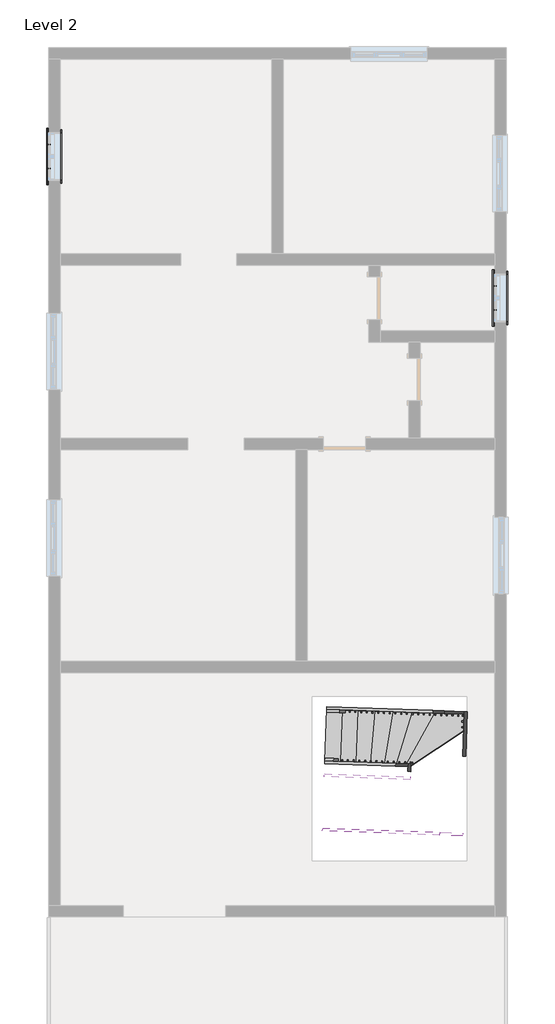
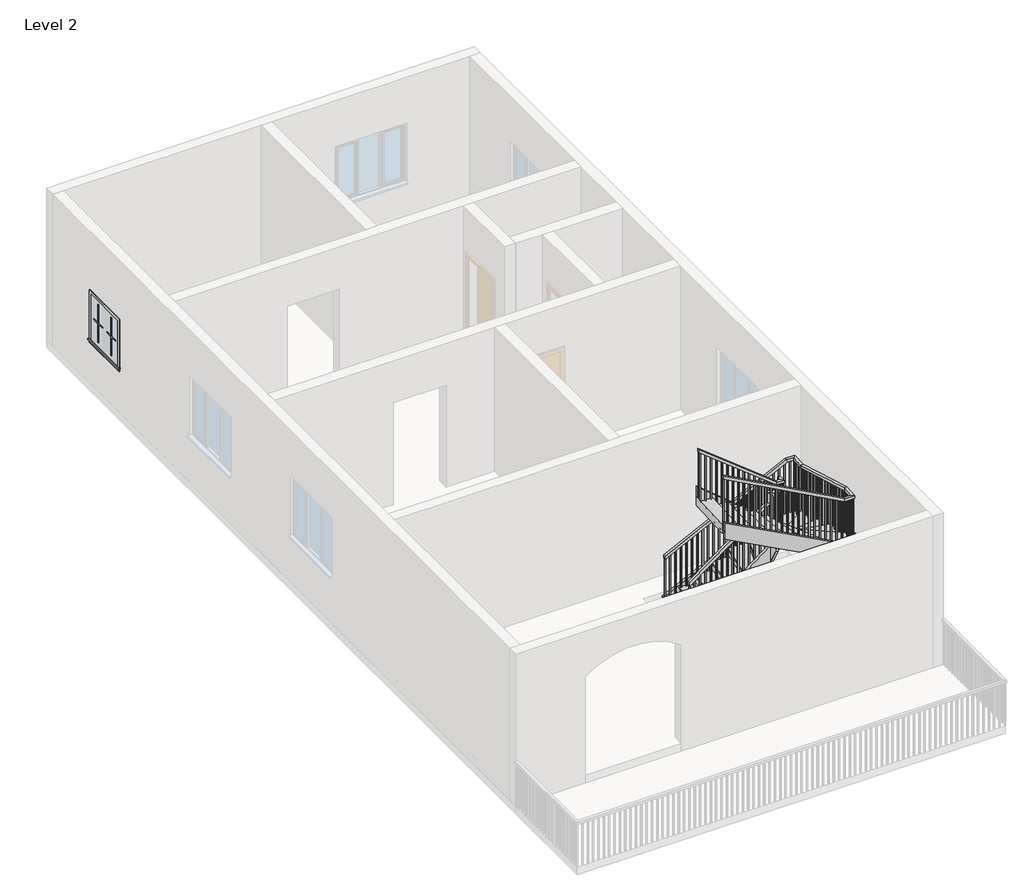
# One storey, part 3 of 3: 8 members, 8 proxies, 2 railings, 1 stair flight.
"""IFC4 building model written with IfcOpenShell, lengths in millimetres."""

from ifc_helpers import new_model, si_unit, frame, origin, place, context, project, spatial, polyline, outline, extrude, faceted_brep, transform, mapped, element, save
from components import muntin_pattern_2x2_muntin_pattern_2x2_b3fe6957, muntin_pattern_2x2_muntin_pattern_2x2_3e0ecaf2, trim_window_exterior_flat_with_sill_41619996, trim_window_interior_flat_picture_frame_51c85655, stair_flight_55d3e88d

model = new_model("IFC4")

# Units and contexts
model_context = context("Model", 3, world=origin())
ifc_project = project(units=[si_unit("LENGTHUNIT", "METRE", prefix="MILLI")], contexts=[model_context])

# Site, building, storey
site = spatial("IfcSite", under=ifc_project)
building = spatial("IfcBuilding", under=site)
storey = spatial("IfcBuildingStorey", under=building, Name="Level 2", Elevation=3048.0)

# Proxies
placement = place(None, origin())
muntin_pattern_2x2_muntin_pattern_2x2_shape = muntin_pattern_2x2_muntin_pattern_2x2_b3fe6957(model_context)
element("IfcBuildingElementProxy", 1, Name="Muntin Pattern_2x2 : Muntin Pattern_2x2", ObjectType="Muntin Pattern_2x2 : Muntin Pattern_2x2", at=placement, inside=storey, context=model_context, shape_type="MappedRepresentation", body=[
    mapped(muntin_pattern_2x2_muntin_pattern_2x2_shape, transform((-14939.9876504, 9248.016357, 4032.25), x_axis=(0.0, 1.0, 0.0), y_axis=(-1.0, 0.0, 0.0), z_axis=(0.0, 0.0, 1.0))),
])
element("IfcBuildingElementProxy", 2, Name="Muntin Pattern_2x2 : Muntin Pattern_2x2", ObjectType="Muntin Pattern_2x2 : Muntin Pattern_2x2", at=placement, inside=storey, context=model_context, shape_type="MappedRepresentation", body=[
    mapped(muntin_pattern_2x2_muntin_pattern_2x2_shape, transform((-7015.1876504, 6733.416357, 4032.25), x_axis=(0.0, 1.0, 0.0), y_axis=(-1.0, 0.0, 0.0), z_axis=(0.0, 0.0, 1.0))),
])
muntin_pattern_2x2_muntin_pattern_2x2_2_shape = muntin_pattern_2x2_muntin_pattern_2x2_3e0ecaf2(model_context)
element("IfcBuildingElementProxy", 3, Name="Muntin Pattern_2x2 : Muntin Pattern_2x2", ObjectType="Muntin Pattern_2x2 : Muntin Pattern_2x2", at=placement, inside=storey, context=model_context, shape_type="MappedRepresentation", body=[
    mapped(muntin_pattern_2x2_muntin_pattern_2x2_2_shape, transform((-14939.9876504, 9676.641357, 4032.25), x_axis=(0.0, -1.0, 0.0), y_axis=(1.0, 0.0, 0.0), z_axis=(0.0, 0.0, 1.0))),
])
element("IfcBuildingElementProxy", 4, Name="Muntin Pattern_2x2 : Muntin Pattern_2x2", ObjectType="Muntin Pattern_2x2 : Muntin Pattern_2x2", at=placement, inside=storey, context=model_context, shape_type="MappedRepresentation", body=[
    mapped(muntin_pattern_2x2_muntin_pattern_2x2_2_shape, transform((-7015.1876504, 7162.041357, 4032.25), x_axis=(0.0, -1.0, 0.0), y_axis=(1.0, 0.0, 0.0), z_axis=(0.0, 0.0, 1.0))),
])
trim_window_exterior_flat_with_sill_shape = trim_window_exterior_flat_with_sill_41619996(model_context)
element("IfcBuildingElementProxy", 5, Name="Trim-Window-Exterior-Flat : with Sill", ObjectType="Trim-Window-Exterior-Flat : with Sill", at=placement, inside=storey, context=model_context, shape_type="MappedRepresentation", body=[
    mapped(trim_window_exterior_flat_with_sill_shape, transform((-14949.5126504, 9462.328857, 4876.8), x_axis=(0.0, -1.0, 0.0), y_axis=(0.0, 0.0, 1.0), z_axis=(-1.0, 0.0, 0.0))),
])
element("IfcBuildingElementProxy", 6, Name="Trim-Window-Exterior-Flat : with Sill", ObjectType="Trim-Window-Exterior-Flat : with Sill", at=placement, inside=storey, context=model_context, shape_type="MappedRepresentation", body=[
    mapped(trim_window_exterior_flat_with_sill_shape, transform((-7024.7126504, 6947.728857, 4876.8), x_axis=(0.0, -1.0, 0.0), y_axis=(0.0, 0.0, 1.0), z_axis=(-1.0, 0.0, 0.0))),
])
trim_window_interior_flat_picture_frame_shape = trim_window_interior_flat_picture_frame_51c85655(model_context)
element("IfcBuildingElementProxy", 7, Name="Trim-Window-Interior-Flat : Picture Frame", ObjectType="Trim-Window-Interior-Flat : Picture Frame", at=placement, inside=storey, context=model_context, shape_type="MappedRepresentation", body=[
    mapped(trim_window_interior_flat_picture_frame_shape, transform((-14746.3126504, 9462.328857, 4876.8), x_axis=(0.0, 1.0, 0.0), y_axis=(0.0, 0.0, 1.0), z_axis=(1.0, 0.0, 0.0))),
])
element("IfcBuildingElementProxy", 8, Name="Trim-Window-Interior-Flat : Picture Frame", ObjectType="Trim-Window-Interior-Flat : Picture Frame", at=placement, inside=storey, context=model_context, shape_type="MappedRepresentation", body=[
    mapped(trim_window_interior_flat_picture_frame_shape, transform((-6821.5126504, 6947.728857, 4876.8), x_axis=(0.0, 1.0, 0.0), y_axis=(0.0, 0.0, 1.0), z_axis=(1.0, 0.0, 0.0))),
])

# Members
element("IfcMember", 9, ObjectType="Stringer - 2\" Width", at=placement, inside=storey, context=model_context, shape_type="SweptSolid", body=[
    extrude(outline(polyline([(157.0794453, -304.8), (51.8818925, -100.6726296), (247.2290139, 0.0), (2348.3102094, 0.0), (2505.3896547, -304.8), (157.0794453, -304.8)])), frame((-10006.394185, -363.3128759, 2934.7449378), z_axis=(0.03595828761805288, 0.9993532916599501, 0.0), x_axis=(0.8883269481492082, -0.03196338688929392, 0.4580977789626134)), (0.0, 0.0, 1.0), 50.8),
])
element("IfcMember", 10, ObjectType="Stringer - 2\" Width", at=placement, inside=storey, context=model_context, shape_type="SweptSolid", body=[
    extrude(outline(polyline([(-7920.3269434, -438.3728236), (-7918.5002624, -387.6056764), (-7564.0151591, -400.3606025), (-7565.8418401, -451.1277497), (-7920.3269434, -438.3728236)])), frame((0.0, 0.0, 4010.500629), z_axis=(0.0, 0.0, 1.0), x_axis=(1.0, 0.0, 0.0)), (0.0, 0.0, 1.0), 342.8950162),
])
element("IfcMember", 11, ObjectType="Stringer - 2\" Width", at=placement, inside=storey, context=model_context, shape_type="SweptSolid", body=[
    extrude(outline(polyline([(-141.4966894, -274.7041443), (-53.351137, 0.0), (2175.2349578, 0.0), (2210.4467651, -11.2985708), (2109.3071449, -326.4985112), (19.9195916, -326.4985112), (-141.4966894, -274.7041443)])), frame((-7515.0746928, -452.9544307, 4353.3956453), z_axis=(-0.9993532916599501, 0.035958287618053086, 0.0), x_axis=(-0.03423883934699899, -0.9515663584286186, 0.3055309597848772)), (0.0, 0.0, 1.0), 50.8),
])
element("IfcMember", 12, ObjectType="Stringer - 2\" Width", at=placement, inside=storey, context=model_context, shape_type="SweptSolid", body=[
    extrude(outline(polyline([(-7590.8819548, -2559.7910402), (-7592.7086358, -2610.5581874), (-7997.9608864, -2595.9765803), (-7996.1342054, -2545.2094331), (-7590.8819548, -2559.7910402)])), frame((0.0, 0.0, 4697.8904473), z_axis=(0.0, 0.0, 1.0), x_axis=(1.0, 0.0, 0.0)), (0.0, 0.0, 1.0), 320.1068224),
])
element("IfcMember", 13, ObjectType="Stringer - 2\" Width", at=placement, inside=storey, context=model_context, shape_type="SweptSolid", body=[
    extrude(outline(polyline([(-146.6402244, -284.5435333), (0.0, 0.0), (2348.3102094, 0.0), (2201.669985, -284.5435333), (-146.6402244, -284.5435333)])), frame((-7997.9608864, -2595.9765803, 5017.9972697), z_axis=(0.03595828761805283, 0.9993532916599502, 0.0), x_axis=(-0.8883269481492087, 0.03196338688929389, 0.45809777896261245)), (0.0, 0.0, 1.0), 50.8),
])
element("IfcMember", 14, ObjectType="Stringer - 2\" Width", at=placement, inside=storey, context=model_context, shape_type="SweptSolid", body=[
    extrude(outline(polyline([(248.5240347, -304.8), (137.1927864, -168.2588219), (343.5522597, 0.0), (1905.6564494, 0.0), (2154.1804842, -304.8), (248.5240347, -304.8)])), frame((-10041.1011242, -1327.888673, 2830.8988904), z_axis=(0.03595828761805293, 0.9993532916599501, 0.0), x_axis=(0.7745239433168307, -0.02786857756239004, 0.6319303787709498)), (0.0, 0.0, 1.0), 50.8),
])
element("IfcMember", 15, ObjectType="Stringer - 2\" Width", at=placement, inside=storey, context=model_context, shape_type="SweptSolid", body=[
    extrude(outline(polyline([(-470.0446027, -275.2513009), (0.0, 0.0), (408.9230004, 1e-07), (420.0212921, -18.9524702), (-68.1184117, -304.7999999), (-452.7413132, -304.8), (-470.0446027, -275.2513009)])), frame((-8512.5307482, -1332.0561414, 4621.2682978), z_axis=(-0.9993532916599503, 0.03595828761805068, 0.0), x_axis=(-0.018170454813323342, -0.5049935642524197, 0.8629318250218347)), (0.0, 0.0, 1.0), 50.8),
])
element("IfcMember", 16, ObjectType="Stringer - 2\" Width", at=placement, inside=storey, context=model_context, shape_type="SweptSolid", body=[
    extrude(outline(polyline([(-248.5240348, -304.8), (0.0, 0.0), (1971.2027087, 0.0), (1722.6786739, -304.8), (-248.5240348, -304.8)])), frame((-8522.5774937, -1611.2754511, 4974.1409689), z_axis=(0.0359582876180528, 0.9993532916599502, 0.0), x_axis=(-0.7745239433168305, 0.027868577562389935, 0.63193037877095)), (0.0, 0.0, 1.0), 50.8),
])

# Railings
element("IfcRailing", 17, ObjectType="Handrail - Rectangular", at=placement, inside=storey, context=model_context, shape_type="SolidModel", body=[
    faceted_brep([(-10037.4477622, -1226.3543786, 4131.7333333), (-10037.4477622, -1226.3543786, 4067.4000346), (-10039.2744432, -1277.1215258, 4067.4000346), (-10039.2744432, -1277.1215258, 4131.7333333), (-8586.854788, -1278.5489726, 5259.6191036), (-8536.0876408, -1280.3756536, 5234.7590024), (-8537.9143218, -1331.1428009, 5234.7590024), (-8588.681469, -1329.3161198, 5259.6191036), (-8586.854788, -1278.5489726, 5462.6281882), (-8536.0876408, -1280.3756536, 5411.8281882), (-8537.9143218, -1331.1428009, 5411.8281882), (-8588.681469, -1329.3161198, 5462.6281882), (-8459.9369199, -1283.1156752, 5462.6281882), (-8459.9369199, -1283.1156752, 5411.8281882), (-8512.5307482, -1332.0561414, 5411.8281882), (-8512.5307482, -1332.0561414, 5462.6281882), (-8464.5036225, -1410.0335432, 5462.6281882), (-8465.5507758, -1439.136044, 5411.8281882), (-8516.317923, -1437.309363, 5411.8281882), (-8515.2707697, -1408.2068622, 5462.6281882), (-8469.070325, -1536.9514112, 5679.5051451), (-8470.897006, -1587.7185585, 5665.7256424), (-8521.6641532, -1585.8918774, 5665.7256424), (-8519.8374722, -1535.1247302, 5679.5051451), (-8469.070325, -1536.9514112, 5882.5142297), (-8470.897006, -1587.7185585, 5831.7142297), (-8521.6641532, -1585.8918774, 5831.7142297), (-8519.8374722, -1535.1247302, 5882.5142297), (-8473.6370275, -1663.8692793, 5882.5142297), (-8473.6370275, -1663.8692793, 5831.7142297), (-8522.5774937, -1611.2754511, 5831.7142297), (-8522.5774937, -1611.2754511, 5882.5142297), (-8600.5548956, -1659.3025768, 5882.5142297), (-8617.9603, -1658.6763032, 5831.7142297), (-8616.133619, -1607.909156, 5831.7142297), (-8598.7282145, -1608.5354295, 5882.5142297), (-10051.1478698, -1607.1079827, 7010.4), (-10049.3211887, -1556.3408355, 7010.4), (-10049.3211887, -1556.3408355, 6946.0667013), (-10051.1478698, -1607.1079827, 6946.0667013)], [[[0, 1, 2, 3]], [[1, 0, 4, 5]], [[2, 1, 5, 6]], [[3, 2, 6, 7]], [[0, 3, 7, 4]], [[5, 4, 8, 9]], [[6, 5, 9, 10]], [[7, 6, 10, 11]], [[4, 7, 11, 8]], [[9, 8, 12, 13]], [[10, 9, 13, 14]], [[11, 10, 14, 15]], [[8, 11, 15, 12]], [[13, 12, 16, 17]], [[14, 13, 17, 18]], [[15, 14, 18, 19]], [[12, 15, 19, 16]], [[17, 16, 20, 21]], [[18, 17, 21, 22]], [[19, 18, 22, 23]], [[16, 19, 23, 20]], [[21, 20, 24, 25]], [[22, 21, 25, 26]], [[23, 22, 26, 27]], [[20, 23, 27, 24]], [[25, 24, 28, 29]], [[26, 25, 29, 30]], [[27, 26, 30, 31]], [[24, 27, 31, 28]], [[29, 28, 32, 33]], [[30, 29, 33, 34]], [[31, 30, 34, 35]], [[28, 31, 35, 32]], [[36, 37, 38, 39]], [[33, 32, 36, 39]], [[34, 33, 39, 38]], [[35, 34, 38, 37]], [[32, 35, 37, 36]]]),
    extrude(outline(polyline([(236.0012245, -19.05), (221.1987754, 0.0), (1225.3637939, 0.0), (1225.3637939, -19.05), (236.0012245, -19.05)])), frame((-10030.9830199, -1591.9482723, 7152.0304606), z_axis=(0.0359582876180528, 0.9993532916599503, 0.0), x_axis=(0.0, 0.0, -1.0)), (0.0, 0.0, 1.0), 19.05),
    extrude(outline(polyline([(236.0012246, -19.05), (221.1987755, 0.0), (1146.417399, 0.0), (1146.417399, -19.05), (236.0012246, -19.05)])), frame((-9929.4487255, -1595.6016343, 7073.0840657), z_axis=(0.0359582876180528, 0.9993532916599503, 0.0), x_axis=(0.0, 0.0, -1.0)), (0.0, 0.0, 1.0), 19.05),
    extrude(outline(polyline([(236.0012245, -19.05), (221.1987755, 0.0), (1067.471004, 0.0), (1067.471004, -19.05), (236.0012245, -19.05)])), frame((-9827.914431, -1599.2549963, 6994.1376707), z_axis=(0.0359582876180528, 0.9993532916599503, 0.0), x_axis=(0.0, 0.0, -1.0)), (0.0, 0.0, 1.0), 19.05),
    extrude(outline(polyline([(236.0012245, -19.05), (221.1987754, 0.0), (1157.8579424, 0.0), (1157.8579424, -19.05), (236.0012245, -19.05)])), frame((-9726.3801366, -1602.9083583, 6915.1912757), z_axis=(0.0359582876180528, 0.9993532916599503, 0.0), x_axis=(0.0, 0.0, -1.0)), (0.0, 0.0, 1.0), 19.05),
    extrude(outline(polyline([(236.0012246, -19.05), (221.1987755, 0.0), (1078.9115475, 0.0), (1078.9115475, -19.05), (236.0012246, -19.05)])), frame((-9624.8458422, -1606.5617203, 6836.2448808), z_axis=(0.0359582876180528, 0.9993532916599503, 0.0), x_axis=(0.0, 0.0, -1.0)), (0.0, 0.0, 1.0), 19.05),
    extrude(outline(polyline([(236.0012245, -19.05), (221.1987755, 0.0), (999.9651525, 0.0), (999.9651525, -19.05), (236.0012245, -19.05)])), frame((-9523.3115477, -1610.2150824, 6757.2984858), z_axis=(0.0359582876180528, 0.9993532916599503, 0.0), x_axis=(0.0, 0.0, -1.0)), (0.0, 0.0, 1.0), 19.05),
    extrude(outline(polyline([(236.0012245, -19.05), (221.1987754, 0.0), (1090.3520908, 0.0), (1090.3520908, -19.05), (236.0012245, -19.05)])), frame((-9421.7772533, -1613.8684444, 6678.3520908), z_axis=(0.0359582876180528, 0.9993532916599503, 0.0), x_axis=(0.0, 0.0, -1.0)), (0.0, 0.0, 1.0), 19.05),
    extrude(outline(polyline([(236.0012246, -19.05), (221.1987755, 0.0), (1011.4056959, 0.0), (1011.4056959, -19.05), (236.0012246, -19.05)])), frame((-9320.2429589, -1617.5218064, 6599.4056959), z_axis=(0.0359582876180528, 0.9993532916599503, 0.0), x_axis=(0.0, 0.0, -1.0)), (0.0, 0.0, 1.0), 19.05),
    extrude(outline(polyline([(236.0012245, -19.05), (221.1987755, 0.0), (1101.7926342, 0.0), (1101.7926342, -19.05), (236.0012245, -19.05)])), frame((-9218.7086644, -1621.1751684, 6520.4593009), z_axis=(0.0359582876180528, 0.9993532916599503, 0.0), x_axis=(0.0, 0.0, -1.0)), (0.0, 0.0, 1.0), 19.05),
    extrude(outline(polyline([(236.0012245, -19.05), (221.1987755, 0.0), (1022.8462392, 0.0), (1022.8462392, -19.05), (236.0012245, -19.05)])), frame((-9117.17437, -1624.8285304, 6441.5129059), z_axis=(0.0359582876180528, 0.9993532916599503, 0.0), x_axis=(0.0, 0.0, -1.0)), (0.0, 0.0, 1.0), 19.05),
    extrude(outline(polyline([(236.0012245, -19.05), (221.1987754, 0.0), (943.8998442, 0.0), (943.8998442, -19.05), (236.0012245, -19.05)])), frame((-9015.6400756, -1628.4818925, 6362.5665109), z_axis=(0.0359582876180528, 0.9993532916599503, 0.0), x_axis=(0.0, 0.0, -1.0)), (0.0, 0.0, 1.0), 19.05),
    extrude(outline(polyline([(236.0012246, -19.05), (221.1987755, 0.0), (1034.2867827, 0.0), (1034.2867827, -19.05), (236.0012246, -19.05)])), frame((-8914.1057811, -1632.1352545, 6283.620116), z_axis=(0.0359582876180528, 0.9993532916599503, 0.0), x_axis=(0.0, 0.0, -1.0)), (0.0, 0.0, 1.0), 19.05),
    extrude(outline(polyline([(236.0012245, -19.05), (221.1987755, 0.0), (955.3403877, 0.0), (955.3403877, -19.05), (236.0012245, -19.05)])), frame((-8812.5714867, -1635.7886165, 6204.673721), z_axis=(0.0359582876180528, 0.9993532916599503, 0.0), x_axis=(0.0, 0.0, -1.0)), (0.0, 0.0, 1.0), 19.05),
    extrude(outline(polyline([(236.0012245, -19.05), (221.1987754, 0.0), (1045.727326, 0.0), (1045.727326, -19.05), (236.0012245, -19.05)])), frame((-8711.0371923, -1639.4419785, 6125.727326), z_axis=(0.0359582876180528, 0.9993532916599503, 0.0), x_axis=(0.0, 0.0, -1.0)), (0.0, 0.0, 1.0), 19.05),
    extrude(outline(polyline([(236.0012246, -19.05), (221.1987755, 0.0), (966.7809311, 0.0), (966.7809311, -19.05), (236.0012246, -19.05)])), frame((-8609.5028978, -1643.0953406, 6046.7809311), z_axis=(0.0359582876180528, 0.9993532916599503, 0.0), x_axis=(0.0, 0.0, -1.0)), (0.0, 0.0, 1.0), 19.05),
    extrude(outline(polyline([(-8506.3702575, -1602.3274488), (-8487.3325773, -1603.0124541), (-8488.0175827, -1622.0501344), (-8507.0552629, -1621.365129), (-8506.3702575, -1602.3274488)])), frame((0.0, 0.0, 4741.3333333), z_axis=(0.0, 0.0, 1.0), x_axis=(1.0, 0.0, 0.0)), (0.0, 0.0, 1.0), 1090.3808964),
    extrude(outline(polyline([(244.8657718, -19.05), (212.3342282, 0.0), (1192.1994682, 0.0), (1192.1994682, -19.05), (244.8657718, -19.05)])), frame((-8484.3642207, -1520.5158399, 5764.1994682), z_axis=(-0.9993532916599502, 0.035958287618050686, 0.0), x_axis=(0.0, 0.0, -1.0)), (0.0, 0.0, 1.0), 19.05),
    extrude(outline(polyline([(244.8657717, -19.05), (212.3342282, 0.0), (1188.0312359, 0.0), (1188.0312359, -19.05), (244.8657717, -19.05)])), frame((-8480.7108586, -1418.9815455, 5590.6979026), z_axis=(-0.9993532916599502, 0.035958287618050686, 0.0), x_axis=(0.0, 0.0, -1.0)), (0.0, 0.0, 1.0), 19.05),
    extrude(outline(polyline([(-8525.208029, -1315.7147199), (-8524.5230236, -1296.6770397), (-8505.4853434, -1297.3620451), (-8506.1703488, -1316.3997253), (-8525.208029, -1315.7147199)])), frame((0.0, 0.0, 4233.3333333), z_axis=(0.0, 0.0, 1.0), x_axis=(1.0, 0.0, 0.0)), (0.0, 0.0, 1.0), 1178.4948549),
    extrude(outline(polyline([(221.1987754, -19.05), (236.0012245, 0.0), (1337.2495642, 0.0), (1337.2495642, -19.05), (221.1987754, -19.05)])), frame((-8626.7423234, -1312.0613579, 5401.2495642), z_axis=(0.035958287618052934, 0.9993532916599503, 0.0), x_axis=(0.0, 0.0, -1.0)), (0.0, 0.0, 1.0), 19.05),
    extrude(outline(polyline([(221.1987755, -19.0500001), (236.0012246, 0.0), (1258.3031693, 0.0), (1258.3031693, -19.0500001), (221.1987755, -19.0500001)])), frame((-8728.2766179, -1308.4079959, 5322.3031693), z_axis=(0.035958287618052934, 0.9993532916599503, 0.0), x_axis=(0.0, 0.0, -1.0)), (0.0, 0.0, 1.0), 19.05),
    extrude(outline(polyline([(221.1987755, -19.05), (236.0012245, 0.0), (1348.6901076, 0.0), (1348.6901076, -19.05), (221.1987755, -19.05)])), frame((-8829.8109123, -1304.7546339, 5243.3567743), z_axis=(0.035958287618052934, 0.9993532916599503, 0.0), x_axis=(0.0, 0.0, -1.0)), (0.0, 0.0, 1.0), 19.05),
    extrude(outline(polyline([(221.1987754, -19.05), (236.0012245, 0.0), (1269.7437126, 0.0), (1269.7437126, -19.05), (221.1987754, -19.05)])), frame((-8931.3452067, -1301.1012718, 5164.4103793), z_axis=(0.035958287618052934, 0.9993532916599503, 0.0), x_axis=(0.0, 0.0, -1.0)), (0.0, 0.0, 1.0), 19.05),
    extrude(outline(polyline([(221.1987755, -19.05), (236.0012246, 0.0), (1360.1306511, 0.0), (1360.1306511, -19.05), (221.1987755, -19.05)])), frame((-9032.8795011, -1297.4479098, 5085.4639844), z_axis=(0.035958287618052934, 0.9993532916599503, 0.0), x_axis=(0.0, 0.0, -1.0)), (0.0, 0.0, 1.0), 19.05),
    extrude(outline(polyline([(221.1987755, -19.05), (236.0012245, 0.0), (1281.1842561, 0.0), (1281.1842561, -19.05), (221.1987755, -19.05)])), frame((-9134.4137956, -1293.7945478, 5006.5175894), z_axis=(0.035958287618052934, 0.9993532916599503, 0.0), x_axis=(0.0, 0.0, -1.0)), (0.0, 0.0, 1.0), 19.05),
    extrude(outline(polyline([(221.1987755, -19.05), (236.0012245, 0.0), (1371.5711944, 0.0), (1371.5711944, -19.05), (221.1987755, -19.05)])), frame((-9235.94809, -1290.1411858, 4927.5711944), z_axis=(0.035958287618052934, 0.9993532916599503, 0.0), x_axis=(0.0, 0.0, -1.0)), (0.0, 0.0, 1.0), 19.05),
    extrude(outline(polyline([(221.1987754, -19.05), (236.0012245, 0.0), (1292.6247994, 0.0), (1292.6247994, -19.05), (221.1987754, -19.05)])), frame((-9337.4823844, -1286.4878237, 4848.6247994), z_axis=(0.035958287618052934, 0.9993532916599503, 0.0), x_axis=(0.0, 0.0, -1.0)), (0.0, 0.0, 1.0), 19.05),
    extrude(outline(polyline([(221.1987755, -19.05), (236.0012246, 0.0), (1213.6784045, 0.0), (1213.6784045, -19.05), (221.1987755, -19.05)])), frame((-9439.0166789, -1282.8344617, 4769.6784045), z_axis=(0.035958287618052934, 0.9993532916599503, 0.0), x_axis=(0.0, 0.0, -1.0)), (0.0, 0.0, 1.0), 19.05),
    extrude(outline(polyline([(221.1987755, -19.05), (236.0012245, 0.0), (1304.0653428, 0.0), (1304.0653428, -19.05), (221.1987755, -19.05)])), frame((-9540.5509733, -1279.1810997, 4690.7320095), z_axis=(0.035958287618052934, 0.9993532916599503, 0.0), x_axis=(0.0, 0.0, -1.0)), (0.0, 0.0, 1.0), 19.05),
    extrude(outline(polyline([(221.1987754, -19.05), (236.0012245, 0.0), (1225.1189478, 0.0), (1225.1189478, -19.05), (221.1987754, -19.05)])), frame((-9642.0852677, -1275.5277377, 4611.7856145), z_axis=(0.035958287618052934, 0.9993532916599503, 0.0), x_axis=(0.0, 0.0, -1.0)), (0.0, 0.0, 1.0), 19.05),
    extrude(outline(polyline([(221.1987755, -19.05), (236.0012246, 0.0), (1146.1725529, 0.0), (1146.1725529, -19.05), (221.1987755, -19.05)])), frame((-9743.6195622, -1271.8743757, 4532.8392196), z_axis=(0.035958287618052934, 0.9993532916599503, 0.0), x_axis=(0.0, 0.0, -1.0)), (0.0, 0.0, 1.0), 19.05),
    extrude(outline(polyline([(221.1987755, -19.05), (236.0012245, 0.0), (1236.5594913, 0.0), (1236.5594913, -19.05), (221.1987755, -19.05)])), frame((-9845.1538566, -1268.2210136, 4453.8928246), z_axis=(0.035958287618052934, 0.9993532916599503, 0.0), x_axis=(0.0, 0.0, -1.0)), (0.0, 0.0, 1.0), 19.05),
    extrude(outline(polyline([(221.1987755, -19.05), (236.0012245, 0.0), (1157.6130963, 0.0), (1157.6130963, -19.05), (221.1987755, -19.05)])), frame((-9946.688151, -1264.5676516, 4374.9464296), z_axis=(0.035958287618052934, 0.9993532916599503, 0.0), x_axis=(0.0, 0.0, -1.0)), (0.0, 0.0, 1.0), 19.05),
    extrude(outline(polyline([(-8507.283598, -1627.7110224), (-8488.2459178, -1628.3960278), (-8488.9309232, -1647.433708), (-8507.9686034, -1646.7487026), (-8507.283598, -1627.7110224)])), frame((0.0, 0.0, 4910.6666667), z_axis=(0.0, 0.0, 1.0), x_axis=(1.0, 0.0, 0.0)), (0.0, 0.0, 1.0), 921.0475631),
    extrude(outline(polyline([(-8496.0951768, -1316.7622457), (-8495.4101715, -1297.7245655), (-8476.3724912, -1298.4095708), (-8477.0574966, -1317.4472511), (-8496.0951768, -1316.7622457)])), frame((0.0, 0.0, 4233.3333333), z_axis=(0.0, 0.0, 1.0), x_axis=(1.0, 0.0, 0.0)), (0.0, 0.0, 1.0), 1178.4948549),
    extrude(outline(polyline([(236.0012245, -19.05), (221.1987755, 0.0), (1240.5988101, 0.0), (1240.5988101, -19.05), (236.0012245, -19.05)])), frame((-10050.5770319, -1591.2432492, 7167.2654768), z_axis=(0.0359582876180528, 0.9993532916599503, 0.0), x_axis=(0.0, 0.0, -1.0)), (0.0, 0.0, 1.0), 19.05),
    extrude(outline(polyline([(221.1987755, -19.05), (236.0012246, 0.0), (1086.0679259, 0.0), (1086.0679259, -19.05), (221.1987755, -19.05)])), frame((-10038.7036054, -1261.2567923, 4303.4012592), z_axis=(0.035958287618052934, 0.9993532916599503, 0.0), x_axis=(0.0, 0.0, -1.0)), (0.0, 0.0, 1.0), 19.05),
])
element("IfcRailing", 18, ObjectType="Handrail - Rectangular", at=placement, inside=storey, context=model_context, shape_type="SolidModel", body=[
    faceted_brep([(-10006.394185, -363.3128759, 4131.7333333), (-10006.394185, -363.3128759, 4074.2742652), (-10008.220866, -414.0800231, 4074.2742652), (-10008.220866, -414.0800231, 4131.7333333), (-7750.1292126, -444.496803, 5325.0239201), (-7737.5382959, -444.9498438, 5274.2239201), (-7739.364977, -495.716991, 5274.2239201), (-7751.9558936, -495.2639503, 5325.0239201), (-7565.8418401, -451.1277497, 5325.0239201), (-7565.8418401, -451.1277497, 5274.2239201), (-7618.4356683, -500.0682159, 5274.2239201), (-7618.4356683, -500.0682159, 5325.0239201), (-7576.1730834, -738.2538248, 5325.0239201), (-7576.4589725, -746.1992592, 5274.2239201), (-7627.2261197, -744.3725782, 5274.2239201), (-7626.9402306, -736.4271438, 5325.0239201), (-7631.3178587, -2270.838284, 5817.1094132), (-7631.6037478, -2278.7837184, 5766.3094132), (-7682.370895, -2276.9570374, 5766.3094132), (-7682.0850059, -2269.011603, 5817.1094132), (-7641.649102, -2557.9643591, 5817.1094132), (-7641.649102, -2557.9643591, 5766.3094132), (-7690.5895682, -2505.3705309, 5766.3094132), (-7690.5895682, -2505.3705309, 5817.1094132), (-7825.9364745, -2551.3334125, 5817.1094132), (-7838.5273911, -2550.8803717, 5766.3094132), (-7836.7007101, -2500.1132245, 5766.3094132), (-7824.1097935, -2500.5662653, 5817.1094132), (-10082.2014469, -2470.1494854, 7010.4), (-10080.3747659, -2419.3823382, 7010.4), (-10080.3747659, -2419.3823382, 6952.9409318), (-10082.2014469, -2470.1494854, 6952.9409318)], [[[0, 1, 2, 3]], [[1, 0, 4, 5]], [[2, 1, 5, 6]], [[3, 2, 6, 7]], [[0, 3, 7, 4]], [[5, 4, 8, 9]], [[6, 5, 9, 10]], [[7, 6, 10, 11]], [[4, 7, 11, 8]], [[9, 8, 12, 13]], [[10, 9, 13, 14]], [[11, 10, 14, 15]], [[8, 11, 15, 12]], [[13, 12, 16, 17]], [[14, 13, 17, 18]], [[15, 14, 18, 19]], [[12, 15, 19, 16]], [[17, 16, 20, 21]], [[18, 17, 21, 22]], [[19, 18, 22, 23]], [[16, 19, 23, 20]], [[21, 20, 24, 25]], [[22, 21, 25, 26]], [[23, 22, 26, 27]], [[20, 23, 27, 24]], [[28, 29, 30, 31]], [[25, 24, 28, 31]], [[26, 25, 31, 30]], [[27, 26, 30, 29]], [[24, 27, 29, 28]]]),
    extrude(outline(polyline([(223.5656878, 19.05), (1212.6274313, 19.05), (1212.6274313, 0.0), (233.6343122, 0.0), (223.5656878, 19.05)])), frame((-9992.2317697, -2457.5014613, 7139.294098), z_axis=(0.035958287618052934, 0.9993532916599503, 0.0), x_axis=(0.0, 0.0, -1.0)), (0.0, 0.0, 1.0), 19.05),
    extrude(outline(polyline([(223.5656878, 19.05), (1158.9281011, 19.05), (1158.9281011, 0.0), (233.6343122, 0.0), (223.5656878, 19.05)])), frame((-9890.6974752, -2461.1548233, 7085.5947678), z_axis=(0.035958287618052934, 0.9993532916599503, 0.0), x_axis=(0.0, 0.0, -1.0)), (0.0, 0.0, 1.0), 19.05),
    extrude(outline(polyline([(223.5656878, 19.05), (1274.5621043, 19.05), (1274.5621043, 0.0), (233.6343122, 0.0), (223.5656878, 19.05)])), frame((-9789.1631808, -2464.8081854, 7031.8954376), z_axis=(0.035958287618052934, 0.9993532916599503, 0.0), x_axis=(0.0, 0.0, -1.0)), (0.0, 0.0, 1.0), 19.05),
    extrude(outline(polyline([(223.5656878, 19.05), (1220.8627741, 19.05), (1220.8627741, 0.0), (233.6343122, 0.0), (223.5656878, 19.05)])), frame((-9687.6288864, -2468.4615474, 6978.1961074), z_axis=(0.035958287618052934, 0.9993532916599503, 0.0), x_axis=(0.0, 0.0, -1.0)), (0.0, 0.0, 1.0), 19.05),
    extrude(outline(polyline([(223.5656878, 19.05), (1167.1634439, 19.05), (1167.1634439, 0.0), (233.6343122, 0.0), (223.5656878, 19.05)])), frame((-9586.0945919, -2472.1149094, 6924.4967772), z_axis=(0.035958287618052934, 0.9993532916599503, 0.0), x_axis=(0.0, 0.0, -1.0)), (0.0, 0.0, 1.0), 19.05),
    extrude(outline(polyline([(223.5656878, 19.05), (1282.797447, 19.05), (1282.797447, 0.0), (233.6343122, 0.0), (223.5656878, 19.05)])), frame((-9484.5602975, -2475.7682714, 6870.797447), z_axis=(0.035958287618052934, 0.9993532916599503, 0.0), x_axis=(0.0, 0.0, -1.0)), (0.0, 0.0, 1.0), 19.05),
    extrude(outline(polyline([(223.5656878, 19.05), (1229.0981168, 19.05), (1229.0981168, 0.0), (233.6343122, 0.0), (223.5656878, 19.05)])), frame((-9383.0260031, -2479.4216334, 6817.0981168), z_axis=(0.035958287618052934, 0.9993532916599503, 0.0), x_axis=(0.0, 0.0, -1.0)), (0.0, 0.0, 1.0), 19.05),
    extrude(outline(polyline([(223.5656878, 19.05), (1175.3987866, 19.05), (1175.3987866, 0.0), (233.6343122, 0.0), (223.5656878, 19.05)])), frame((-9281.4917086, -2483.0749955, 6763.3987866), z_axis=(0.035958287618052934, 0.9993532916599503, 0.0), x_axis=(0.0, 0.0, -1.0)), (0.0, 0.0, 1.0), 19.05),
    extrude(outline(polyline([(223.5656878, 19.05), (1291.0327897, 19.05), (1291.0327897, 0.0), (233.6343122, 0.0), (223.5656878, 19.05)])), frame((-9179.9574142, -2486.7283575, 6709.6994564), z_axis=(0.035958287618052934, 0.9993532916599503, 0.0), x_axis=(0.0, 0.0, -1.0)), (0.0, 0.0, 1.0), 19.05),
    extrude(outline(polyline([(223.5656878, 19.05), (1237.3334595, 19.05), (1237.3334595, 0.0), (233.6343122, 0.0), (223.5656878, 19.05)])), frame((-9078.4231198, -2490.3817195, 6656.0001262), z_axis=(0.035958287618052934, 0.9993532916599503, 0.0), x_axis=(0.0, 0.0, -1.0)), (0.0, 0.0, 1.0), 19.05),
    extrude(outline(polyline([(223.5656878, 19.05), (1183.6341293, 19.05), (1183.6341293, 0.0), (233.6343122, 0.0), (223.5656878, 19.05)])), frame((-8976.8888253, -2494.0350815, 6602.300796), z_axis=(0.035958287618052934, 0.9993532916599503, 0.0), x_axis=(0.0, 0.0, -1.0)), (0.0, 0.0, 1.0), 19.05),
    extrude(outline(polyline([(223.5656878, 19.05), (1299.2681325, 19.05), (1299.2681325, 0.0), (233.6343122, 0.0), (223.5656878, 19.05)])), frame((-8875.3545309, -2497.6884436, 6548.6014658), z_axis=(0.035958287618052934, 0.9993532916599503, 0.0), x_axis=(0.0, 0.0, -1.0)), (0.0, 0.0, 1.0), 19.05),
    extrude(outline(polyline([(223.5656878, 19.05), (1245.5688023, 19.05), (1245.5688023, 0.0), (233.6343122, 0.0), (223.5656878, 19.05)])), frame((-8773.8202365, -2501.3418056, 6494.9021356), z_axis=(0.035958287618052934, 0.9993532916599503, 0.0), x_axis=(0.0, 0.0, -1.0)), (0.0, 0.0, 1.0), 19.05),
    extrude(outline(polyline([(223.5656878, 19.05), (1191.8694721, 19.05), (1191.8694721, 0.0), (233.6343122, 0.0), (223.5656878, 19.05)])), frame((-8672.285942, -2504.9951676, 6441.2028054), z_axis=(0.035958287618052934, 0.9993532916599503, 0.0), x_axis=(0.0, 0.0, -1.0)), (0.0, 0.0, 1.0), 19.05),
    extrude(outline(polyline([(223.5656878, 19.05), (1138.1701419, 19.05), (1138.1701419, 0.0), (233.6343122, 0.0), (223.5656878, 19.05)])), frame((-8570.7516476, -2508.6485296, 6387.5034752), z_axis=(0.035958287618052934, 0.9993532916599503, 0.0), x_axis=(0.0, 0.0, -1.0)), (0.0, 0.0, 1.0), 19.05),
    extrude(outline(polyline([(223.5656878, 19.05), (1253.804145, 19.05), (1253.804145, 0.0), (233.6343122, 0.0), (223.5656878, 19.05)])), frame((-8469.2173532, -2512.3018916, 6333.804145), z_axis=(0.035958287618052934, 0.9993532916599503, 0.0), x_axis=(0.0, 0.0, -1.0)), (0.0, 0.0, 1.0), 19.05),
    extrude(outline(polyline([(223.5656878, 19.05), (1200.1048148, 19.05), (1200.1048148, 0.0), (233.6343122, 0.0), (223.5656878, 19.05)])), frame((-8367.6830587, -2515.9552537, 6280.1048148), z_axis=(0.035958287618052934, 0.9993532916599503, 0.0), x_axis=(0.0, 0.0, -1.0)), (0.0, 0.0, 1.0), 19.05),
    extrude(outline(polyline([(223.5656878, 19.05), (1146.4054846, 19.05), (1146.4054846, 0.0), (233.6343122, 0.0), (223.5656878, 19.05)])), frame((-8266.1487643, -2519.6086157, 6226.4054846), z_axis=(0.035958287618052934, 0.9993532916599503, 0.0), x_axis=(0.0, 0.0, -1.0)), (0.0, 0.0, 1.0), 19.05),
    extrude(outline(polyline([(223.5656878, 19.05), (1092.7061544, 19.05), (1092.7061544, 0.0), (233.6343122, 0.0), (223.5656878, 19.05)])), frame((-8164.6144699, -2523.2619777, 6172.7061544), z_axis=(0.035958287618052934, 0.9993532916599503, 0.0), x_axis=(0.0, 0.0, -1.0)), (0.0, 0.0, 1.0), 19.05),
    extrude(outline(polyline([(223.5656878, 19.05), (1208.3401575, 19.05), (1208.3401575, 0.0), (233.6343122, 0.0), (223.5656878, 19.05)])), frame((-8063.0801754, -2526.9153397, 6119.0068242), z_axis=(0.035958287618052934, 0.9993532916599503, 0.0), x_axis=(0.0, 0.0, -1.0)), (0.0, 0.0, 1.0), 19.05),
    extrude(outline(polyline([(223.5656878, 19.05), (1154.6408273, 19.05), (1154.6408273, 0.0), (233.6343122, 0.0), (223.5656878, 19.05)])), frame((-7961.545881, -2530.5687018, 6065.307494), z_axis=(0.035958287618052934, 0.9993532916599503, 0.0), x_axis=(0.0, 0.0, -1.0)), (0.0, 0.0, 1.0), 19.05),
    extrude(outline(polyline([(223.5656878, 19.05), (1100.9414971, 19.05), (1100.9414971, 0.0), (233.6343122, 0.0), (223.5656878, 19.05)])), frame((-7860.0115866, -2534.2220638, 6011.6081638), z_axis=(0.035958287618052934, 0.9993532916599503, 0.0), x_axis=(0.0, 0.0, -1.0)), (0.0, 0.0, 1.0), 19.05),
    extrude(outline(polyline([(-7758.4772921, -2537.8754258), (-7777.5149723, -2537.1904204), (-7776.829967, -2518.1527402), (-7757.7922868, -2518.8377456), (-7758.4772921, -2537.8754258)])), frame((0.0, 0.0, 4910.6666667), z_axis=(0.0, 0.0, 1.0), x_axis=(1.0, 0.0, 0.0)), (0.0, 0.0, 1.0), 855.6427466),
    extrude(outline(polyline([(-7655.3446518, -2497.107534), (-7656.0296572, -2516.1452142), (-7675.0673374, -2515.4602088), (-7674.382332, -2496.4225286), (-7655.3446518, -2497.107534)])), frame((0.0, 0.0, 4910.6666667), z_axis=(0.0, 0.0, 1.0), x_axis=(1.0, 0.0, 0.0)), (0.0, 0.0, 1.0), 855.6427466),
    extrude(outline(polyline([(-7651.6912898, -2395.5732396), (-7652.3762952, -2414.6109198), (-7671.4139754, -2413.9259144), (-7670.72897, -2394.8882342), (-7651.6912898, -2395.5732396)])), frame((0.0, 0.0, 4910.6666667), z_axis=(0.0, 0.0, 1.0), x_axis=(1.0, 0.0, 0.0)), (0.0, 0.0, 1.0), 855.6427466),
    extrude(outline(polyline([(-7648.0379278, -2294.0389451), (-7648.7229332, -2313.0766254), (-7667.7606134, -2312.39162), (-7667.075608, -2293.3539398), (-7648.0379278, -2294.0389451)])), frame((0.0, 0.0, 4910.6666667), z_axis=(0.0, 0.0, 1.0), x_axis=(1.0, 0.0, 0.0)), (0.0, 0.0, 1.0), 855.6427466),
    extrude(outline(polyline([(225.5436705, 19.05), (1229.1130279, 19.05), (1229.1130279, 0.0), (231.6563296, 0.0), (225.5436705, 19.05)])), frame((-7644.3845658, -2192.5046507, 5970.4463612), z_axis=(-0.9993532916599501, 0.03595828761805307, 0.0), x_axis=(0.0, 0.0, -1.0)), (0.0, 0.0, 1.0), 19.05),
    extrude(outline(polyline([(225.5436704, 19.05), (1196.5121796, 19.05), (1196.5121796, 0.0), (231.6563295, 0.0), (225.5436704, 19.05)])), frame((-7640.7312037, -2090.9703563, 5937.8455129), z_axis=(-0.9993532916599501, 0.03595828761805307, 0.0), x_axis=(0.0, 0.0, -1.0)), (0.0, 0.0, 1.0), 19.05),
    extrude(outline(polyline([(225.5436705, 19.0500001), (1163.9113314, 19.0500001), (1163.9113314, 0.0), (231.6563295, 0.0), (225.5436705, 19.0500001)])), frame((-7637.0778417, -1989.4360618, 5905.2446647), z_axis=(-0.9993532916599501, 0.03595828761805307, 0.0), x_axis=(0.0, 0.0, -1.0)), (0.0, 0.0, 1.0), 19.05),
    extrude(outline(polyline([(225.5436705, 19.05), (1131.3104832, 19.05), (1131.3104832, 0.0), (231.6563295, 0.0), (225.5436705, 19.05)])), frame((-7633.4244797, -1887.9017674, 5872.6438165), z_axis=(-0.9993532916599501, 0.03595828761805307, 0.0), x_axis=(0.0, 0.0, -1.0)), (0.0, 0.0, 1.0), 19.05),
    extrude(outline(polyline([(225.5436705, 19.05), (1098.709635, 19.05), (1098.709635, 0.0), (231.6563296, 0.0), (225.5436705, 19.05)])), frame((-7629.7711177, -1786.367473, 5840.0429683), z_axis=(-0.9993532916599501, 0.03595828761805307, 0.0), x_axis=(0.0, 0.0, -1.0)), (0.0, 0.0, 1.0), 19.05),
    extrude(outline(polyline([(225.5436705, 19.0500001), (1235.44212, 19.0500001), (1235.44212, 0.0), (231.6563295, 0.0), (225.5436705, 19.0500001)])), frame((-7626.1177556, -1684.8331785, 5807.44212), z_axis=(-0.9993532916599501, 0.03595828761805307, 0.0), x_axis=(0.0, 0.0, -1.0)), (0.0, 0.0, 1.0), 19.05),
    extrude(outline(polyline([(225.5436705, 19.05), (1202.8412718, 19.05), (1202.8412718, 0.0), (231.6563295, 0.0), (225.5436705, 19.05)])), frame((-7622.4643936, -1583.2988841, 5774.8412718), z_axis=(-0.9993532916599501, 0.03595828761805307, 0.0), x_axis=(0.0, 0.0, -1.0)), (0.0, 0.0, 1.0), 19.05),
    extrude(outline(polyline([(225.5436705, 19.05), (1170.2404236, 19.05), (1170.2404236, 0.0), (231.6563296, 0.0), (225.5436705, 19.05)])), frame((-7618.8110316, -1481.7645897, 5742.2404236), z_axis=(-0.9993532916599501, 0.03595828761805307, 0.0), x_axis=(0.0, 0.0, -1.0)), (0.0, 0.0, 1.0), 19.05),
    extrude(outline(polyline([(225.5436704, 19.05), (1137.6395753, 19.05), (1137.6395753, 0.0), (231.6563295, 0.0), (225.5436704, 19.05)])), frame((-7615.1576696, -1380.2302953, 5709.6395753), z_axis=(-0.9993532916599501, 0.03595828761805307, 0.0), x_axis=(0.0, 0.0, -1.0)), (0.0, 0.0, 1.0), 19.05),
    extrude(outline(polyline([(225.5436705, 19.05), (1105.0387271, 19.05), (1105.0387271, 0.0), (231.6563295, 0.0), (225.5436705, 19.05)])), frame((-7611.5043076, -1278.6960008, 5677.0387271), z_axis=(-0.9993532916599501, 0.03595828761805307, 0.0), x_axis=(0.0, 0.0, -1.0)), (0.0, 0.0, 1.0), 19.05),
    extrude(outline(polyline([(225.5436705, 19.05), (1241.7712122, 19.05), (1241.7712122, 0.0), (231.6563295, 0.0), (225.5436705, 19.05)])), frame((-7607.8509455, -1177.1617064, 5644.4378789), z_axis=(-0.9993532916599501, 0.03595828761805307, 0.0), x_axis=(0.0, 0.0, -1.0)), (0.0, 0.0, 1.0), 19.05),
    extrude(outline(polyline([(225.5436705, 19.05), (1209.170364, 19.05), (1209.170364, 0.0), (231.6563296, 0.0), (225.5436705, 19.05)])), frame((-7604.1975835, -1075.627412, 5611.8370307), z_axis=(-0.9993532916599501, 0.03595828761805307, 0.0), x_axis=(0.0, 0.0, -1.0)), (0.0, 0.0, 1.0), 19.05),
    extrude(outline(polyline([(225.5436704, 19.05), (1176.5695157, 19.05), (1176.5695157, 0.0), (231.6563295, 0.0), (225.5436704, 19.05)])), frame((-7600.5442215, -974.0931175, 5579.2361824), z_axis=(-0.9993532916599501, 0.03595828761805307, 0.0), x_axis=(0.0, 0.0, -1.0)), (0.0, 0.0, 1.0), 19.05),
    extrude(outline(polyline([(225.5436705, 19.05), (1143.9686675, 19.05), (1143.9686675, 0.0), (231.6563295, 0.0), (225.5436705, 19.05)])), frame((-7596.8908595, -872.5588231, 5546.6353342), z_axis=(-0.9993532916599501, 0.03595828761805307, 0.0), x_axis=(0.0, 0.0, -1.0)), (0.0, 0.0, 1.0), 19.05),
    extrude(outline(polyline([(225.5436705, 19.05), (1111.3678193, 19.05), (1111.3678193, 0.0), (231.6563295, 0.0), (225.5436705, 19.05)])), frame((-7593.2374974, -771.0245287, 5514.034486), z_axis=(-0.9993532916599501, 0.03595828761805307, 0.0), x_axis=(0.0, 0.0, -1.0)), (0.0, 0.0, 1.0), 19.05),
    extrude(outline(polyline([(-7589.5841354, -669.4902342), (-7590.2691408, -688.5279144), (-7609.306821, -687.842909), (-7608.6218156, -668.8052288), (-7589.5841354, -669.4902342)])), frame((0.0, 0.0, 4233.3333333), z_axis=(0.0, 0.0, 1.0), x_axis=(1.0, 0.0, 0.0)), (0.0, 0.0, 1.0), 1040.8905868),
    extrude(outline(polyline([(-7585.9307734, -567.9559398), (-7586.6157788, -586.99362), (-7605.653459, -586.3086146), (-7604.9684536, -567.2709344), (-7585.9307734, -567.9559398)])), frame((0.0, 0.0, 4233.3333333), z_axis=(0.0, 0.0, 1.0), x_axis=(1.0, 0.0, 0.0)), (0.0, 0.0, 1.0), 1040.8905868),
    extrude(outline(polyline([(-7681.195091, -462.8624332), (-7662.1574108, -463.5474386), (-7662.8424161, -482.5851188), (-7681.8800963, -481.9001134), (-7681.195091, -462.8624332)])), frame((0.0, 0.0, 4233.3333333), z_axis=(0.0, 0.0, 1.0), x_axis=(1.0, 0.0, 0.0)), (0.0, 0.0, 1.0), 1040.8905868),
    extrude(outline(polyline([(233.6343122, 19.05), (1250.9261963, 19.05), (1250.9261963, 0.0), (223.5656878, 0.0), (233.6343122, 19.05)])), frame((-7764.3767106, -478.9317568, 5484.2595296), z_axis=(0.03595828761805286, 0.9993532916599503, 0.0), x_axis=(0.0, 0.0, -1.0)), (0.0, 0.0, 1.0), 19.05),
    extrude(outline(polyline([(233.6343122, 19.05), (1197.2268661, 19.05), (1197.2268661, 0.0), (223.5656878, 0.0), (233.6343122, 19.05)])), frame((-7865.911005, -475.2783948, 5430.5601994), z_axis=(0.03595828761805286, 0.9993532916599503, 0.0), x_axis=(0.0, 0.0, -1.0)), (0.0, 0.0, 1.0), 19.05),
    extrude(outline(polyline([(233.6343122, 19.05), (1143.5275359, 19.05), (1143.5275359, 0.0), (223.5656878, 0.0), (233.6343122, 19.05)])), frame((-7967.4452994, -471.6250327, 5376.8608692), z_axis=(0.03595828761805286, 0.9993532916599503, 0.0), x_axis=(0.0, 0.0, -1.0)), (0.0, 0.0, 1.0), 19.05),
    extrude(outline(polyline([(233.6343122, 19.05), (1089.8282057, 19.05), (1089.8282057, 0.0), (223.5656878, 0.0), (233.6343122, 19.05)])), frame((-8068.9795939, -467.9716707, 5323.161539), z_axis=(0.03595828761805286, 0.9993532916599503, 0.0), x_axis=(0.0, 0.0, -1.0)), (0.0, 0.0, 1.0), 19.05),
    extrude(outline(polyline([(233.6343122, 19.05), (1205.4622088, 19.05), (1205.4622088, 0.0), (223.5656878, 0.0), (233.6343122, 19.05)])), frame((-8170.5138883, -464.3183087, 5269.4622088), z_axis=(0.03595828761805286, 0.9993532916599503, 0.0), x_axis=(0.0, 0.0, -1.0)), (0.0, 0.0, 1.0), 19.05),
    extrude(outline(polyline([(233.6343122, 19.05), (1151.7628786, 19.05), (1151.7628786, 0.0), (223.5656878, 0.0), (233.6343122, 19.05)])), frame((-8272.0481827, -460.6649467, 5215.7628786), z_axis=(0.03595828761805286, 0.9993532916599503, 0.0), x_axis=(0.0, 0.0, -1.0)), (0.0, 0.0, 1.0), 19.05),
    extrude(outline(polyline([(233.6343122, 19.05), (1098.0635484, 19.05), (1098.0635484, 0.0), (223.5656878, 0.0), (233.6343122, 19.05)])), frame((-8373.5824772, -457.0115846, 5162.0635484), z_axis=(0.03595828761805286, 0.9993532916599503, 0.0), x_axis=(0.0, 0.0, -1.0)), (0.0, 0.0, 1.0), 19.05),
    extrude(outline(polyline([(233.6343122, 19.05), (1044.3642182, 19.05), (1044.3642182, 0.0), (223.5656878, 0.0), (233.6343122, 19.05)])), frame((-8475.1167716, -453.3582226, 5108.3642182), z_axis=(0.03595828761805286, 0.9993532916599503, 0.0), x_axis=(0.0, 0.0, -1.0)), (0.0, 0.0, 1.0), 19.05),
    extrude(outline(polyline([(233.6343122, 19.05), (1159.9982213, 19.05), (1159.9982213, 0.0), (223.5656878, 0.0), (233.6343122, 19.05)])), frame((-8576.651066, -449.7048606, 5054.664888), z_axis=(0.03595828761805286, 0.9993532916599503, 0.0), x_axis=(0.0, 0.0, -1.0)), (0.0, 0.0, 1.0), 19.05),
    extrude(outline(polyline([(233.6343122, 19.05), (1106.2988911, 19.05), (1106.2988911, 0.0), (223.5656878, 0.0), (233.6343122, 19.05)])), frame((-8678.1853605, -446.0514986, 5000.9655578), z_axis=(0.03595828761805286, 0.9993532916599503, 0.0), x_axis=(0.0, 0.0, -1.0)), (0.0, 0.0, 1.0), 19.05),
    extrude(outline(polyline([(233.6343122, 19.05), (1052.5995609, 19.05), (1052.5995609, 0.0), (223.5656878, 0.0), (233.6343122, 19.05)])), frame((-8779.7196549, -442.3981366, 4947.2662276), z_axis=(0.03595828761805286, 0.9993532916599503, 0.0), x_axis=(0.0, 0.0, -1.0)), (0.0, 0.0, 1.0), 19.05),
    extrude(outline(polyline([(233.6343122, 19.05), (1168.2335641, 19.05), (1168.2335641, 0.0), (223.5656878, 0.0), (233.6343122, 19.05)])), frame((-8881.2539493, -438.7447745, 4893.5668974), z_axis=(0.03595828761805286, 0.9993532916599503, 0.0), x_axis=(0.0, 0.0, -1.0)), (0.0, 0.0, 1.0), 19.05),
    extrude(outline(polyline([(233.6343122, 19.05), (1114.5342339, 19.05), (1114.5342339, 0.0), (223.5656878, 0.0), (233.6343122, 19.05)])), frame((-8982.7882438, -435.0914125, 4839.8675672), z_axis=(0.03595828761805286, 0.9993532916599503, 0.0), x_axis=(0.0, 0.0, -1.0)), (0.0, 0.0, 1.0), 19.05),
    extrude(outline(polyline([(233.6343122, 19.05), (1060.8349037, 19.05), (1060.8349037, 0.0), (223.5656878, 0.0), (233.6343122, 19.05)])), frame((-9084.3225382, -431.4380505, 4786.168237), z_axis=(0.03595828761805286, 0.9993532916599503, 0.0), x_axis=(0.0, 0.0, -1.0)), (0.0, 0.0, 1.0), 19.05),
    extrude(outline(polyline([(233.6343122, 19.05), (1176.4689068, 19.05), (1176.4689068, 0.0), (223.5656878, 0.0), (233.6343122, 19.05)])), frame((-9185.8568326, -427.7846885, 4732.4689068), z_axis=(0.03595828761805286, 0.9993532916599503, 0.0), x_axis=(0.0, 0.0, -1.0)), (0.0, 0.0, 1.0), 19.05),
    extrude(outline(polyline([(233.6343122, 19.05), (1122.7695766, 19.05), (1122.7695766, 0.0), (223.5656878, 0.0), (233.6343122, 19.05)])), frame((-9287.3911271, -424.1313264, 4678.7695766), z_axis=(0.03595828761805286, 0.9993532916599503, 0.0), x_axis=(0.0, 0.0, -1.0)), (0.0, 0.0, 1.0), 19.05),
    extrude(outline(polyline([(233.6343122, 19.05), (1069.0702464, 19.05), (1069.0702464, 0.0), (223.5656878, 0.0), (233.6343122, 19.05)])), frame((-9388.9254215, -420.4779644, 4625.0702464), z_axis=(0.03595828761805286, 0.9993532916599503, 0.0), x_axis=(0.0, 0.0, -1.0)), (0.0, 0.0, 1.0), 19.05),
    extrude(outline(polyline([(233.6343122, 19.05), (1184.7042495, 19.05), (1184.7042495, 0.0), (223.5656878, 0.0), (233.6343122, 19.05)])), frame((-9490.4597159, -416.8246024, 4571.3709162), z_axis=(0.03595828761805286, 0.9993532916599503, 0.0), x_axis=(0.0, 0.0, -1.0)), (0.0, 0.0, 1.0), 19.05),
    extrude(outline(polyline([(233.6343122, 19.05), (1131.0049193, 19.05), (1131.0049193, 0.0), (223.5656878, 0.0), (233.6343122, 19.05)])), frame((-9591.9940104, -413.1712404, 4517.671586), z_axis=(0.03595828761805286, 0.9993532916599503, 0.0), x_axis=(0.0, 0.0, -1.0)), (0.0, 0.0, 1.0), 19.05),
    extrude(outline(polyline([(233.6343122, 19.05), (1077.3055891, 19.05), (1077.3055891, 0.0), (223.5656878, 0.0), (233.6343122, 19.05)])), frame((-9693.5283048, -409.5178784, 4463.9722558), z_axis=(0.03595828761805286, 0.9993532916599503, 0.0), x_axis=(0.0, 0.0, -1.0)), (0.0, 0.0, 1.0), 19.05),
    extrude(outline(polyline([(233.6343122, 19.05), (1192.9395923, 19.05), (1192.9395923, 0.0), (223.5656878, 0.0), (233.6343122, 19.05)])), frame((-9795.0625992, -405.8645163, 4410.2729256), z_axis=(0.03595828761805286, 0.9993532916599503, 0.0), x_axis=(0.0, 0.0, -1.0)), (0.0, 0.0, 1.0), 19.05),
    extrude(outline(polyline([(233.6343123, 19.0500001), (1139.2402621, 19.0500001), (1139.2402621, 0.0), (223.5656878, 0.0), (233.6343123, 19.0500001)])), frame((-9896.5968936, -402.2111543, 4356.5735954), z_axis=(0.03595828761805286, 0.9993532916599503, 0.0), x_axis=(0.0, 0.0, -1.0)), (0.0, 0.0, 1.0), 19.05),
    extrude(outline(polyline([(-7656.2579923, -2522.4911076), (-7656.9429977, -2541.5287878), (-7675.9806779, -2540.8437824), (-7675.2956725, -2521.8061022), (-7656.2579923, -2522.4911076)])), frame((0.0, 0.0, 4910.6666667), z_axis=(0.0, 0.0, 1.0), x_axis=(1.0, 0.0, 0.0)), (0.0, 0.0, 1.0), 855.6427466),
    extrude(outline(polyline([(-7601.3150916, -465.73664), (-7582.2774114, -466.4216454), (-7582.9624168, -485.4593256), (-7602.000097, -484.7743202), (-7601.3150916, -465.73664)])), frame((0.0, 0.0, 4233.3333333), z_axis=(0.0, 0.0, 1.0), x_axis=(1.0, 0.0, 0.0)), (0.0, 0.0, 1.0), 1040.8905868),
    extrude(outline(polyline([(223.5656878, 19.05), (1249.8399529, 19.05), (1249.8399529, 0.0), (233.6343122, 0.0), (223.5656878, 19.05)])), frame((-10062.5929289, -2454.9697572, 7176.5066196), z_axis=(0.035958287618052934, 0.9993532916599503, 0.0), x_axis=(0.0, 0.0, -1.0)), (0.0, 0.0, 1.0), 19.05),
    extrude(outline(polyline([(233.6343122, 19.05), (1090.5752441, 19.05), (1090.5752441, 0.0), (223.5656878, 0.0), (233.6343122, 19.05)])), frame((-9988.612348, -398.900295, 4307.9085774), z_axis=(0.03595828761805286, 0.9993532916599503, 0.0), x_axis=(0.0, 0.0, -1.0)), (0.0, 0.0, 1.0), 19.05),
])

# Stair flight
stair_flight_shape = stair_flight_55d3e88d(model_context)
element("IfcStairFlight", 19, ObjectType="2\" Tread 1\" Nosing 1/4\" Riser", at=placement, inside=storey, context=model_context, shape_type="MappedRepresentation", body=[
    mapped(stair_flight_shape, transform((0.0, 0.0, 0.0), x_axis=(1.0, 0.0, 0.0), y_axis=(0.0, 1.0, 0.0), z_axis=(0.0, 0.0, 1.0))),
])

save(model, "model.ifc")

# Revit data of these elements
# Type "Muntin Pattern_2x2 : Muntin Pattern_2x2"
#   Width [instance default] = 4' - 0"
#   Thickness = 0' - 0 1/2"
#   Height [instance default] = 4' - 0"
#   Distance = 0' - 0 3/4"
#   Interior Material [instance default] = none
#   Exterior Material [instance default] = none
#   Default Elevation = 0
# Type "Trim-Window-Exterior-Flat : with Sill"
#   Trim Width = 0' - 2 1/4"
#   Trim Thickness_Picture Frame = 0' - 1 1/4"
#   Trim Thickness_with Sill = 0' - 0 3/4"
#   Sill Thickness = 0' - 1 1/4"
#   Opening Width [instance default] = 2' - 0"
#   Opening Height [instance default] = 3' - 0"
#   Default Elevation = 4' - 0"
#   Sill = yes
#   Picture Frame = no
#   Trim Material [instance default] = none
# Type "Trim-Window-Interior-Flat : Picture Frame"
#   Trim Thickness_Picture Frame = 0' - 1 1/4"
#   Trim Width = 0' - 2 1/4"
#   Trim Thickness_with Sill = 0' - 0 3/4"
#   Sill Thickness = 0' - 1 1/4"
#   Opening Width [instance default] = 2' - 0"
#   Opening Height [instance default] = 3' - 0"
#   Default Elevation = 4' - 0"
#   Sill = no
#   Picture Frame = yes
#   Trim Material [instance default] = none
# Type "Handrail - Rectangular"
#   Assembly Code = "C2010400"
#   built-in parameter 1008612 = 0.0416667 (stored number, unit not read)
#   built-in parameter 1008611 = 0.0416667 (stored number, unit not read)
#   built-in parameter 1008609 = 0.333333 (stored number, unit not read)
#   built-in parameter 1008604 = 0.166667 (stored number, unit not read)
#   built-in parameter 1008603 = 0.166667 (stored number, unit not read)
#   Railing Height = 3' - 0"
#   built-in parameter 1008630 = 2
#   built-in parameter 1008610 = 2
#   built-in parameter 1008618 = Baluster - Square : 3/4"
# Elements 1, 2, 3, 4 (IfcBuildingElementProxy, "Muntin Pattern_2x2 : Muntin Pattern_2x2")
#   Width = 0' - 11 5/8"
#   Height = 2' - 6 1/2"
#   Interior Material = Wood - Stained
#   Exterior Material = Clad - White
#   Phase Created = New Construction
#   Materials on its faces: "Clad - White", "Wood - Stained"
# Elements 5, 6 (IfcBuildingElementProxy, "Trim-Window-Exterior-Flat : with Sill")
#   Opening Width = 2' - 10"
#   Opening Height = 3' - 0"
#   Trim Material = Clad - White
#   Phase Created = New Construction
#   Materials on its faces: "Clad - White"
# Elements 7, 8 (IfcBuildingElementProxy, "Trim-Window-Interior-Flat : Picture Frame")
#   Opening Width = 2' - 10"
#   Opening Height = 3' - 0"
#   Trim Material = Wood - Stained
#   Phase Created = New Construction
#   Materials on its faces: "Wood - Stained"
# Elements 9, 10, 11, 12, 13, 14, 15, 16 (IfcMember, "Stringer - 2\" Width")
#   Phase Created = New Construction
# Elements 17, 18 (IfcRailing, "Handrail - Rectangular")
#   Phase Created = New Construction
# Element 19 (IfcStairFlight, "2\" Tread 1\" Nosing 1/4\" Riser")
#   Phase Created = New Construction
# Materials
#   "Clad - White": class "Wood", colour RGB 242 242 238, transparency 0, Cost = 0
#   "Wood - Stained": class "Wood", colour RGB 224 178 126, transparency 0, Cost = 0
